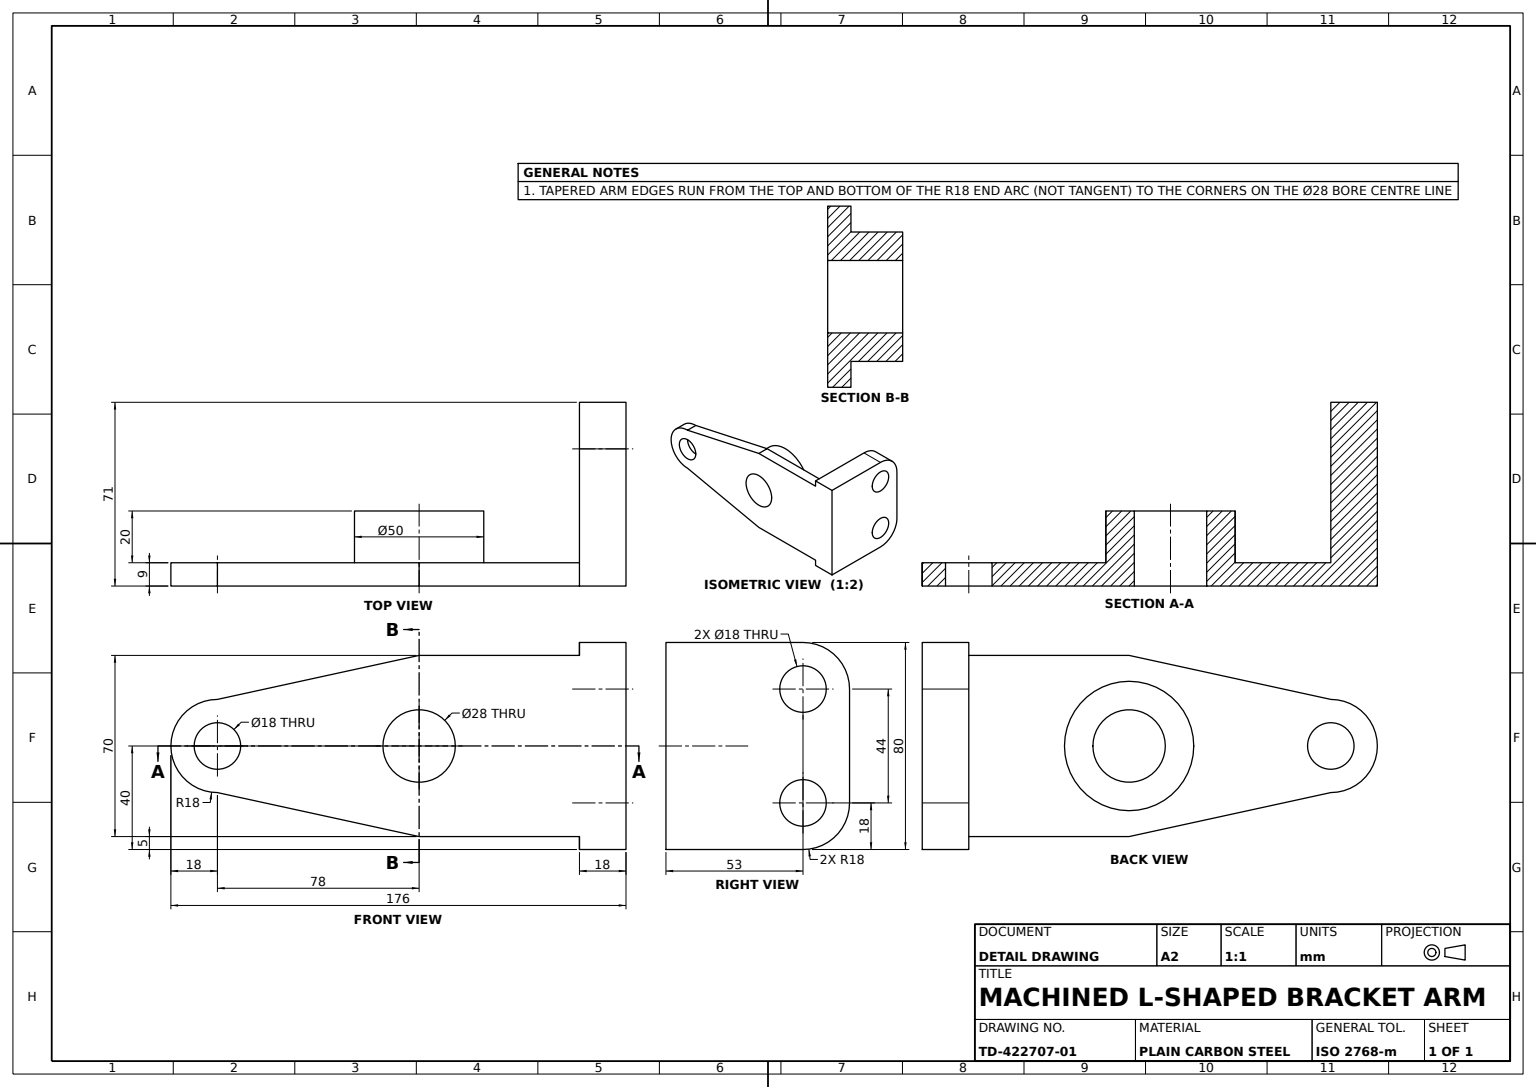
SolidWorks part; units mm, degrees
material "Plain Carbon Steel"
ref_plane "Front Plane" through (0, 0, 0) normal (0, 0, 1) x (1, 0, 0)
ref_plane "Top Plane" through (0, 0, 0) normal (0, 1, 0) x (1, 0, 0)
ref_plane "Right Plane" through (0, 0, 0) normal (1, 0, 0) x (0, 0, -1)
sketch "Base Plate Profile Sketch" plane through (0, 0, 0) normal (0, 0, 1) x (1, 0, 0)
  line L1 (0, 70) -> (69.753, 70)
  line L2 (0, 0) -> (69.753, 0)
  line L3 (80, 75) -> (80, -5)
  line L4 (80.2285, 72.2582) -> (80.2285, -7.7418)
  line L5 (-78, 53) -> (0, 70)
  line L7 (-78, 17) -> (0, 0)
  arc A0 (69.753, 0) -> (80, -5) centre (69.753, -13) cw
  arc A1 (69.753, 70) -> (80, 75) centre (69.753, 83) ccw
  arc A2 (-78, 53) -> (-78, 17) centre (-78, 35) ccw
  point P15 (80, 35)
  dimension "D3" = 13
  dimension "13" = 13
  dimension "D6" = 36
  dimension "D7" = 78
  dimension "D1" = 80
  dimension "D2" = 70
  dimension "D4" = 80
  dimension "D5" = 78
  dimension "D8" = 79.8311
  dimension "D9" = 80.2285
  dimension "D10" = 7.7418
extrude "Base Plate" add sketch "Base Plate Profile Sketch" along normal blind 9 contours L5 A2 L7 L2 A0 L3 A1 L1
sketch "Pivot Axis Reference Sketch" plane through (0, 0, 0) normal (0, 0, -1) x (-1, 0, 0)
  line L0 (0, 70) -> (0, 0) construction
sketch "End Hole Ø18 Sketch" plane through (0, 0, 0) normal (0, 0, -1) x (-1, 0, 0)
  circle A0 centre (78, 35) radius 9
  dimension "D1" = 18
extrude "End Hole Ø18" cut sketch "End Hole Ø18 Sketch" against normal blind 9
sketch "Pivot Boss Ø50 Sketch" plane through (0, 0, 0) normal (0, 0, -1) x (-1, 0, 0)
  line L0 (0, 70) -> (0, 0) construction
  circle A0 centre (0, 35) radius 25
  dimension "D1" = 50
extrude "Pivot Boss Ø50" add sketch "Pivot Boss Ø50 Sketch" along normal blind 20
sketch "Pivot Bore Ø28 Sketch" plane through (0, 0, -20) normal (0, 0, -1) x (-1, 0, 0)
  line L1 (0, 70) -> (0, 0) construction
  circle A0 centre (0, 35) radius 14
  dimension "D1" = 28
extrude "Pivot Bore Ø28" cut sketch "Pivot Bore Ø28 Sketch" against normal through all
sketch "Mounting Block Sketch" plane through (80, 0, 0) normal (1, 0, 0) x (0, 0, -1)
  line L0 (-9, 75) -> (44, 75)
  line L1 (62, 57) -> (62, 13)
  line L2 (44, -5) -> (-9, -5)
  line L3 (-9, -5) -> (-9, 75)
  arc A0 (44, 75) -> (62, 57) centre (44, 57) cw
  arc A1 (62, 13) -> (44, -5) centre (44, 13) cw
  dimension "D1" = 18
  dimension "D2" = 53
extrude "Mounting Block" add sketch "Mounting Block Sketch" against normal blind 18
sketch "Mounting Holes 2xØ18 Sketch" plane through (80, 0, 0) normal (1, 0, 0) x (0, 0, -1)
  circle A0 centre (44, 57) radius 9
  circle A1 centre (44, 13) radius 9
  dimension "D1" = 18
  dimension "D2" = 18
extrude "Mounting Holes 2xØ18" cut sketch "Mounting Holes 2xØ18 Sketch" against normal blind 18
ref_plane "Plane1" through (0, 30, 0) normal (0, 1, 0) x (1, 0, 0)
